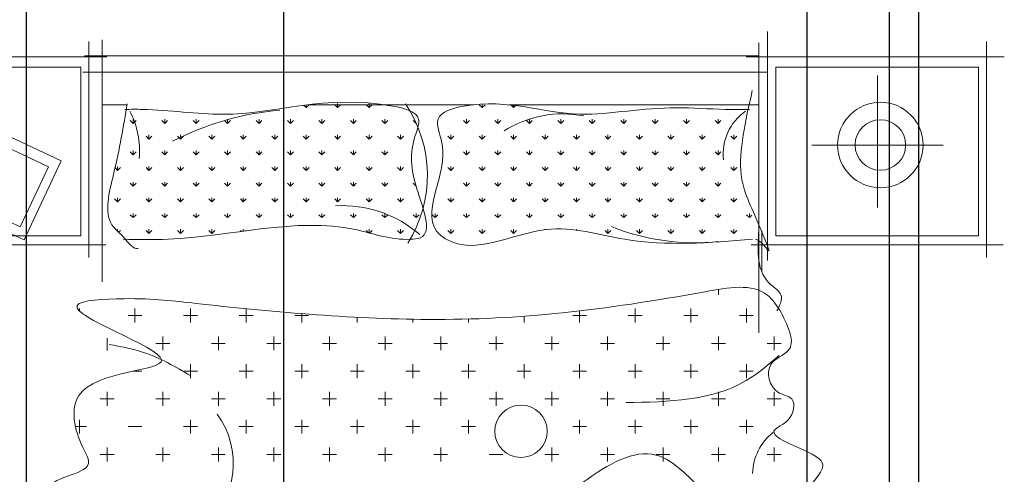
# Model space of a CAD drawing. Units: inches. Extents: x -438 to 102, y -60 to 1091.
# Tile 17 of 20: x -68 to 20, y 766 to 807. Entities that reach past the tile are written whole.
import ezdxf

# ---------------------------------------------------------------- set-up
doc = ezdxf.new("R2010")
doc.units = ezdxf.units.IN
doc.header["$MEASUREMENT"] = 0
doc.layers.add('A-ANNO-DIMS', color=217, linetype='Continuous', lineweight=18, true_color=0x93278f)
doc.layers.add('Furniture', color=7, linetype='Continuous', lineweight=15)
doc.styles.get("Standard").update_dxf_attribs({"font": 'arial.ttf'})
doc.dimstyles.get("Standard").update_dxf_attribs({"dimtxt": 8, "dimasz": 0.18, "dimexe": 0.18, "dimexo": 0.0625, "dimgap": 0.09, "dimtad": 0, "dimtih": 1, "dimtoh": 1, "dimdec": 4, "dimzin": 0, "dimdsep": 46, "dimlunit": 3, "dimtxsty": 'Standard', "dimcen": 0.09, "dimadec": 0, "dimazin": 0, "dimtfac": 1, "dimtdec": 4, "dimtofl": 0, "dimtmove": 0, "dimatfit": 3, "dimfxl": 1, "dimtolj": 1, "dimtzin": 0, "dimarcsym": 0})

# ---------------------------------------------------------------- blocks, each defined once
blk = doc.blocks.new('BED-DOUBLE-WITH-NIGHTSTANDS')
for p, q in [((30.685, 0.003), (30.685, -20.597)), ((-29.157, -22.53), (-29.157, -0.743)), ((-30.374, -20.327), (-30.374, -0.897)), ((29.898, -1.014), (29.898, -27.125)), ((50.37, -20.327), (50.37, -0.897)), ((-28.759, -2.28), (-51.984, -2.28)), ((-30.745, -2.188), (29.898, -2.188)), ((51.985, -2.28), (28.76, -2.28)), ((-31.095, -3.205), (-49.317, -3.205)), ((-31.095, -18.39), (-31.095, -3.205)), ((49.649, -3.205), (31.427, -3.205)), ((31.427, -3.205), (31.427, -18.39)), ((49.649, -18.39), (49.649, -3.205)), ((30.685, -3.641), (-30.922, -3.641)), ((40.583, -3.955), (40.583, -15.85)), ((-26.928, -6.593), (-29.157, -6.593)), ((-10.816, -6.85), (-11.024, -6.642)), ((-10.816, -6.85), (-10.551, -6.585)), ((-10.816, -6.851), (-10.816, -6.616)), ((4.241, -6.593), (-10.627, -6.593)), ((-7.988, -6.85), (-8.253, -6.585)), ((-7.988, -6.85), (-7.723, -6.585)), ((-7.987, -6.851), (-7.987, -6.476)), ((-5.159, -6.85), (-5.425, -6.585)), ((-5.159, -6.851), (-5.159, -6.476)), ((-5.159, -6.85), (-4.894, -6.585)), ((5.018, -6.85), (4.753, -6.585)), ((5.018, -6.851), (5.018, -6.53)), ((5.018, -6.85), (5.283, -6.585)), ((29.898, -6.593), (7.41, -6.593)), ((7.846, -6.85), (7.61, -6.614)), ((7.846, -6.85), (8.033, -6.663)), ((7.847, -6.851), (7.847, -6.641)), ((-26.372, -8.265), (-26.372, -7.89)), ((-23.544, -8.265), (-23.544, -7.89)), ((-20.715, -8.265), (-20.715, -7.89)), ((-17.887, -8.265), (-17.887, -7.89)), ((-15.058, -8.265), (-15.058, -7.89)), ((-12.23, -8.265), (-12.23, -7.89)), ((-9.402, -8.265), (-9.402, -7.89)), ((-6.573, -8.265), (-6.573, -7.89)), ((-3.745, -8.265), (-3.745, -7.89)), ((3.604, -8.265), (3.604, -7.89)), ((6.433, -8.265), (6.433, -7.89)), ((9.261, -8.265), (9.261, -7.89)), ((12.089, -8.265), (12.089, -7.89)), ((14.918, -8.265), (14.918, -7.89)), ((17.746, -8.265), (17.746, -7.89)), ((20.575, -8.265), (20.575, -7.89)), ((23.403, -8.265), (23.403, -7.89)), ((26.232, -8.265), (26.232, -7.89)), ((-26.373, -8.265), (-26.638, -8)), ((-26.373, -8.265), (-26.107, -8)), ((-23.544, -8.265), (-23.809, -8)), ((-23.544, -8.265), (-23.279, -8)), ((-20.716, -8.265), (-20.981, -8)), ((-20.716, -8.265), (-20.451, -8)), ((-17.887, -8.265), (-18.152, -8)), ((-17.887, -8.265), (-17.622, -8)), ((-15.059, -8.265), (-15.324, -8)), ((-15.059, -8.265), (-14.794, -8)), ((-12.23, -8.265), (-12.496, -8)), ((-12.23, -8.265), (-11.965, -8)), ((-9.402, -8.265), (-9.667, -8)), ((-9.402, -8.265), (-9.137, -8)), ((-6.574, -8.265), (-6.839, -8)), ((-6.574, -8.265), (-6.308, -8)), ((-3.745, -8.265), (-4.01, -8)), ((-3.745, -8.265), (-3.48, -8)), ((-0.917, -8.265), (-1.182, -8)), ((-0.917, -8.265), (-0.915, -8.262)), ((-0.916, -8.265), (-0.916, -8.258)), ((1.02, -8.021), (1.041, -8)), ((3.604, -8.265), (3.339, -8)), ((3.604, -8.265), (3.869, -8)), ((6.432, -8.265), (6.167, -8)), ((6.432, -8.265), (6.697, -8)), ((9.261, -8.265), (8.996, -8)), ((9.261, -8.265), (9.526, -8)), ((12.089, -8.265), (11.824, -8)), ((12.089, -8.265), (12.354, -8)), ((14.918, -8.265), (14.652, -8)), ((14.918, -8.265), (15.183, -8)), ((17.746, -8.265), (17.481, -8)), ((17.746, -8.265), (18.011, -8)), ((20.574, -8.265), (20.309, -8)), ((20.574, -8.265), (20.84, -8)), ((23.403, -8.265), (23.138, -8)), ((23.403, -8.265), (23.668, -8)), ((26.231, -8.265), (25.966, -8)), ((26.231, -8.265), (26.496, -8)), ((-32.845, -11.63), (-38.006, -9.214)), ((-24.958, -9.679), (-25.224, -9.414)), ((-24.958, -9.679), (-24.958, -9.304)), ((-24.958, -9.679), (-24.693, -9.414)), ((-22.13, -9.679), (-22.395, -9.414)), ((-22.13, -9.679), (-22.13, -9.304)), ((-22.13, -9.679), (-21.865, -9.414)), ((-19.302, -9.679), (-19.567, -9.414)), ((-19.302, -9.679), (-19.036, -9.414)), ((-19.301, -9.679), (-19.301, -9.304)), ((-16.473, -9.679), (-16.738, -9.414)), ((-16.473, -9.679), (-16.473, -9.304)), ((-16.473, -9.679), (-16.208, -9.414)), ((-13.645, -9.679), (-13.91, -9.414)), ((-13.645, -9.679), (-13.38, -9.414)), ((-13.644, -9.679), (-13.644, -9.304)), ((-10.816, -9.679), (-11.081, -9.414)), ((-10.816, -9.679), (-10.816, -9.304)), ((-10.816, -9.679), (-10.551, -9.414)), ((-7.988, -9.679), (-8.253, -9.414)), ((-7.988, -9.679), (-7.723, -9.414)), ((-7.987, -9.679), (-7.987, -9.304)), ((-5.159, -9.679), (-5.425, -9.414)), ((-5.159, -9.679), (-5.159, -9.304)), ((-5.159, -9.679), (-4.894, -9.414)), ((-2.331, -9.679), (-2.596, -9.414)), ((-2.331, -9.679), (-2.331, -9.304)), ((-2.331, -9.679), (-2.066, -9.414)), ((2.19, -9.679), (1.924, -9.414)), ((2.19, -9.679), (2.19, -9.304)), ((2.19, -9.679), (2.455, -9.414)), ((5.018, -9.679), (4.753, -9.414)), ((5.018, -9.679), (5.018, -9.304)), ((5.018, -9.679), (5.283, -9.414)), ((7.846, -9.679), (7.581, -9.414)), ((7.846, -9.679), (8.112, -9.414)), ((7.847, -9.679), (7.847, -9.304)), ((10.675, -9.679), (10.41, -9.414)), ((10.675, -9.679), (10.675, -9.304)), ((10.675, -9.679), (10.94, -9.414)), ((13.503, -9.679), (13.238, -9.414)), ((13.503, -9.679), (13.768, -9.414)), ((13.504, -9.679), (13.504, -9.304)), ((16.332, -9.679), (16.067, -9.414)), ((16.332, -9.679), (16.332, -9.304)), ((16.332, -9.679), (16.597, -9.414)), ((19.16, -9.679), (18.895, -9.414)), ((19.16, -9.679), (19.425, -9.414)), ((19.161, -9.679), (19.161, -9.304)), ((21.989, -9.679), (21.723, -9.414)), ((21.989, -9.679), (21.989, -9.304)), ((21.989, -9.679), (22.254, -9.414)), ((24.817, -9.679), (24.552, -9.414)), ((24.817, -9.679), (24.817, -9.304)), ((24.817, -9.679), (25.082, -9.414)), ((27.645, -9.679), (27.38, -9.414)), ((27.645, -9.679), (27.911, -9.414)), ((27.646, -9.679), (27.646, -9.304)), ((-34.001, -12.162), (-37.855, -10.358)), ((46.482, -10.214), (34.684, -10.214)), ((-26.373, -11.093), (-26.638, -10.828)), ((-26.373, -11.093), (-26.107, -10.828)), ((-26.372, -11.093), (-26.372, -10.718)), ((-23.544, -11.093), (-23.809, -10.828)), ((-23.544, -11.093), (-23.544, -10.718)), ((-23.544, -11.093), (-23.279, -10.828)), ((-20.716, -11.093), (-20.981, -10.828)), ((-20.716, -11.093), (-20.451, -10.828)), ((-20.715, -11.093), (-20.715, -10.718)), ((-17.887, -11.093), (-18.152, -10.828)), ((-17.887, -11.093), (-17.887, -10.718)), ((-17.887, -11.093), (-17.622, -10.828)), ((-15.059, -11.093), (-15.324, -10.828)), ((-15.059, -11.093), (-14.794, -10.828)), ((-15.058, -11.093), (-15.058, -10.718)), ((-12.23, -11.093), (-12.496, -10.828)), ((-12.23, -11.093), (-12.23, -10.718)), ((-12.23, -11.093), (-11.965, -10.828)), ((-9.402, -11.093), (-9.667, -10.828)), ((-9.402, -11.093), (-9.402, -10.718)), ((-9.402, -11.093), (-9.137, -10.828)), ((-6.574, -11.093), (-6.839, -10.828)), ((-6.574, -11.093), (-6.308, -10.828)), ((-6.573, -11.093), (-6.573, -10.718)), ((-3.745, -11.093), (-4.01, -10.828)), ((-3.745, -11.093), (-3.745, -10.718)), ((-3.745, -11.093), (-3.48, -10.828)), ((3.604, -11.093), (3.339, -10.828)), ((3.604, -11.093), (3.604, -10.718)), ((3.604, -11.093), (3.869, -10.828)), ((6.432, -11.093), (6.167, -10.828)), ((6.432, -11.093), (6.697, -10.828)), ((6.433, -11.093), (6.433, -10.718)), ((9.261, -11.093), (8.996, -10.828)), ((9.261, -11.093), (9.261, -10.718)), ((9.261, -11.093), (9.526, -10.828)), ((12.089, -11.093), (11.824, -10.828)), ((12.089, -11.093), (12.089, -10.718)), ((12.089, -11.093), (12.354, -10.828)), ((14.918, -11.093), (14.652, -10.828)), ((14.918, -11.093), (14.918, -10.718)), ((14.918, -11.093), (15.183, -10.828)), ((17.746, -11.093), (17.481, -10.828)), ((17.746, -11.093), (17.746, -10.718)), ((17.746, -11.093), (18.011, -10.828)), ((20.574, -11.093), (20.309, -10.828)), ((20.574, -11.093), (20.84, -10.828)), ((20.575, -11.093), (20.575, -10.718)), ((23.403, -11.093), (23.138, -10.828)), ((23.403, -11.093), (23.403, -10.718)), ((23.403, -11.093), (23.668, -10.828)), ((26.231, -11.093), (25.966, -10.828)), ((26.231, -11.093), (26.496, -10.828)), ((26.232, -11.093), (26.232, -10.718)), ((-36.532, -17.571), (-34.001, -12.162)), ((-36.181, -18.757), (-32.845, -11.63)), ((-27.787, -12.507), (-28.013, -12.281)), ((-27.787, -12.507), (-27.522, -12.242)), ((-27.786, -12.508), (-27.786, -12.133)), ((-24.958, -12.507), (-25.224, -12.242)), ((-24.958, -12.508), (-24.958, -12.133)), ((-24.958, -12.507), (-24.693, -12.242)), ((-22.13, -12.507), (-22.395, -12.242)), ((-22.13, -12.508), (-22.13, -12.133)), ((-22.13, -12.507), (-21.865, -12.242)), ((-19.302, -12.507), (-19.567, -12.242)), ((-19.302, -12.507), (-19.036, -12.242)), ((-19.301, -12.508), (-19.301, -12.133)), ((-16.473, -12.507), (-16.738, -12.242)), ((-16.473, -12.508), (-16.473, -12.133)), ((-16.473, -12.507), (-16.208, -12.242)), ((-13.645, -12.507), (-13.91, -12.242)), ((-13.645, -12.507), (-13.38, -12.242)), ((-13.644, -12.508), (-13.644, -12.133)), ((-10.816, -12.507), (-11.081, -12.242)), ((-10.816, -12.508), (-10.816, -12.133)), ((-10.816, -12.507), (-10.551, -12.242)), ((-7.988, -12.507), (-8.253, -12.242)), ((-7.988, -12.507), (-7.723, -12.242)), ((-7.987, -12.508), (-7.987, -12.133)), ((-5.159, -12.507), (-5.425, -12.242)), ((-5.159, -12.508), (-5.159, -12.133)), ((-5.159, -12.507), (-4.894, -12.242)), ((-2.331, -12.507), (-2.596, -12.242)), ((-2.331, -12.508), (-2.331, -12.133)), ((-2.331, -12.507), (-2.066, -12.242)), ((2.19, -12.507), (1.924, -12.242)), ((2.19, -12.508), (2.19, -12.133)), ((2.19, -12.507), (2.455, -12.242)), ((5.018, -12.507), (4.753, -12.242)), ((5.018, -12.508), (5.018, -12.133)), ((5.018, -12.507), (5.283, -12.242)), ((7.846, -12.507), (7.581, -12.242)), ((7.846, -12.507), (8.112, -12.242)), ((7.847, -12.508), (7.847, -12.133)), ((10.675, -12.507), (10.41, -12.242)), ((10.675, -12.508), (10.675, -12.133)), ((10.675, -12.507), (10.94, -12.242)), ((13.503, -12.507), (13.238, -12.242)), ((13.503, -12.507), (13.768, -12.242)), ((13.504, -12.508), (13.504, -12.133)), ((16.332, -12.507), (16.067, -12.242)), ((16.332, -12.508), (16.332, -12.133)), ((16.332, -12.507), (16.597, -12.242)), ((19.16, -12.507), (18.895, -12.242)), ((19.16, -12.507), (19.425, -12.242)), ((19.161, -12.508), (19.161, -12.133)), ((21.989, -12.507), (21.723, -12.242)), ((21.989, -12.508), (21.989, -12.133)), ((21.989, -12.507), (22.254, -12.242)), ((24.817, -12.507), (24.552, -12.242)), ((24.817, -12.508), (24.817, -12.133)), ((24.817, -12.507), (25.082, -12.242)), ((27.645, -12.507), (27.38, -12.242)), ((27.645, -12.507), (27.911, -12.242)), ((27.646, -12.508), (27.646, -12.133)), ((-26.373, -13.922), (-26.638, -13.656)), ((-26.373, -13.922), (-26.107, -13.656)), ((-26.372, -13.922), (-26.372, -13.547)), ((-23.544, -13.922), (-23.809, -13.656)), ((-23.544, -13.922), (-23.544, -13.547)), ((-23.544, -13.922), (-23.279, -13.656)), ((-20.716, -13.922), (-20.981, -13.656)), ((-20.716, -13.922), (-20.451, -13.656)), ((-20.715, -13.922), (-20.715, -13.547)), ((-17.887, -13.922), (-18.152, -13.656)), ((-17.887, -13.922), (-17.887, -13.547)), ((-17.887, -13.922), (-17.622, -13.656)), ((-15.059, -13.922), (-15.324, -13.656)), ((-15.059, -13.922), (-14.794, -13.656)), ((-15.058, -13.922), (-15.058, -13.547)), ((-12.23, -13.922), (-12.496, -13.656)), ((-12.23, -13.922), (-12.23, -13.547)), ((-12.23, -13.922), (-11.965, -13.656)), ((-9.402, -13.922), (-9.667, -13.656)), ((-9.402, -13.922), (-9.402, -13.547)), ((-9.402, -13.922), (-9.137, -13.656)), ((-6.574, -13.922), (-6.839, -13.656)), ((-6.574, -13.922), (-6.308, -13.656)), ((-6.573, -13.922), (-6.573, -13.547)), ((-3.745, -13.922), (-4.01, -13.656)), ((-3.745, -13.922), (-3.745, -13.547)), ((-3.745, -13.922), (-3.48, -13.656)), ((-0.933, -13.906), (-1.182, -13.656)), ((1.022, -13.675), (1.041, -13.656)), ((3.604, -13.922), (3.339, -13.656)), ((3.604, -13.922), (3.604, -13.547)), ((3.604, -13.922), (3.869, -13.656)), ((6.432, -13.922), (6.167, -13.656)), ((6.432, -13.922), (6.697, -13.656)), ((6.433, -13.922), (6.433, -13.547)), ((9.261, -13.922), (8.996, -13.656)), ((9.261, -13.922), (9.261, -13.547)), ((9.261, -13.922), (9.526, -13.656)), ((12.089, -13.922), (11.824, -13.656)), ((12.089, -13.922), (12.089, -13.547)), ((12.089, -13.922), (12.354, -13.656)), ((14.918, -13.922), (14.652, -13.656)), ((14.918, -13.922), (14.918, -13.547)), ((14.918, -13.922), (15.183, -13.656)), ((17.746, -13.922), (17.481, -13.656)), ((17.746, -13.922), (17.746, -13.547)), ((17.746, -13.922), (18.011, -13.656)), ((20.574, -13.922), (20.309, -13.656)), ((20.574, -13.922), (20.84, -13.656)), ((20.575, -13.922), (20.575, -13.547)), ((23.403, -13.922), (23.138, -13.656)), ((23.403, -13.922), (23.403, -13.547)), ((23.403, -13.922), (23.668, -13.656)), ((26.231, -13.922), (25.966, -13.656)), ((26.231, -13.922), (26.496, -13.656)), ((26.232, -13.922), (26.232, -13.547)), ((-27.786, -15.336), (-27.786, -14.961)), ((-24.958, -15.336), (-24.958, -14.961)), ((-22.13, -15.336), (-22.13, -14.961)), ((-19.301, -15.336), (-19.301, -14.961)), ((-16.473, -15.336), (-16.473, -14.961)), ((-13.644, -15.336), (-13.644, -14.961)), ((-10.816, -15.336), (-10.816, -14.961)), ((-7.987, -15.336), (-7.987, -14.961)), ((-5.159, -15.336), (-5.159, -14.961)), ((-2.331, -15.336), (-2.331, -14.961)), ((2.19, -15.336), (2.19, -14.961)), ((5.018, -15.336), (5.018, -14.961)), ((7.847, -15.336), (7.847, -14.961)), ((10.675, -15.336), (10.675, -14.961)), ((13.504, -15.336), (13.504, -14.961)), ((16.332, -15.336), (16.332, -14.961)), ((19.161, -15.336), (19.161, -14.961)), ((21.989, -15.336), (21.989, -14.961)), ((24.817, -15.336), (24.817, -14.961)), ((27.646, -15.336), (27.646, -14.961)), ((-40.387, -15.767), (-36.532, -17.571)), ((-27.787, -15.336), (-28.052, -15.071)), ((-27.787, -15.336), (-27.522, -15.071)), ((-24.958, -15.336), (-25.224, -15.071)), ((-24.958, -15.336), (-24.693, -15.071)), ((-22.13, -15.336), (-22.395, -15.071)), ((-22.13, -15.336), (-21.865, -15.071)), ((-19.302, -15.336), (-19.567, -15.071)), ((-19.302, -15.336), (-19.036, -15.071)), ((-16.473, -15.336), (-16.738, -15.071)), ((-16.473, -15.336), (-16.208, -15.071)), ((-13.645, -15.336), (-13.91, -15.071)), ((-13.645, -15.336), (-13.38, -15.071)), ((-10.816, -15.336), (-11.081, -15.071)), ((-10.816, -15.336), (-10.551, -15.071)), ((-7.988, -15.336), (-8.253, -15.071)), ((-7.988, -15.336), (-7.723, -15.071)), ((-5.159, -15.336), (-5.425, -15.071)), ((-5.159, -15.336), (-4.894, -15.071)), ((-2.331, -15.336), (-2.596, -15.071)), ((-2.331, -15.336), (-2.066, -15.071)), ((2.19, -15.336), (1.924, -15.071)), ((2.19, -15.336), (2.455, -15.071)), ((5.018, -15.336), (4.753, -15.071)), ((5.018, -15.336), (5.283, -15.071)), ((7.846, -15.336), (7.581, -15.071)), ((7.846, -15.336), (8.112, -15.071)), ((10.675, -15.336), (10.41, -15.071)), ((10.675, -15.336), (10.94, -15.071)), ((13.503, -15.336), (13.238, -15.071)), ((13.503, -15.336), (13.768, -15.071)), ((16.332, -15.336), (16.067, -15.071)), ((16.332, -15.336), (16.597, -15.071)), ((19.16, -15.336), (18.895, -15.071)), ((19.16, -15.336), (19.425, -15.071)), ((21.989, -15.336), (21.723, -15.071)), ((21.989, -15.336), (22.254, -15.071)), ((24.817, -15.336), (24.552, -15.071)), ((24.817, -15.336), (25.082, -15.071)), ((27.645, -15.336), (27.38, -15.071)), ((27.645, -15.336), (27.911, -15.071)), ((-41.342, -16.341), (-36.181, -18.757)), ((-26.373, -16.75), (-26.638, -16.485)), ((-26.373, -16.75), (-26.107, -16.485)), ((-26.372, -16.75), (-26.372, -16.375)), ((-23.544, -16.75), (-23.809, -16.485)), ((-23.544, -16.75), (-23.544, -16.375)), ((-23.544, -16.75), (-23.279, -16.485)), ((-20.716, -16.75), (-20.981, -16.485)), ((-20.716, -16.75), (-20.451, -16.485)), ((-20.715, -16.75), (-20.715, -16.375)), ((-17.887, -16.75), (-18.152, -16.485)), ((-17.887, -16.75), (-17.887, -16.375)), ((-17.887, -16.75), (-17.622, -16.485)), ((-15.059, -16.75), (-15.324, -16.485)), ((-15.059, -16.75), (-14.794, -16.485)), ((-15.058, -16.75), (-15.058, -16.375)), ((-12.23, -16.75), (-12.496, -16.485)), ((-12.23, -16.75), (-12.23, -16.375)), ((-12.23, -16.75), (-11.965, -16.485)), ((-9.402, -16.75), (-9.667, -16.485)), ((-9.402, -16.75), (-9.402, -16.375)), ((-9.402, -16.75), (-9.137, -16.485)), ((-6.574, -16.75), (-6.839, -16.485)), ((-6.574, -16.75), (-6.308, -16.485)), ((-6.573, -16.75), (-6.573, -16.375)), ((-3.745, -16.75), (-4.01, -16.485)), ((-3.745, -16.75), (-3.745, -16.375)), ((-3.745, -16.75), (-3.48, -16.485)), ((-0.917, -16.75), (-1.182, -16.485)), ((-0.917, -16.75), (-0.652, -16.485)), ((-0.916, -16.75), (-0.916, -16.375)), ((0.775, -16.75), (0.51, -16.485)), ((0.775, -16.75), (1.041, -16.485)), ((0.776, -16.75), (0.776, -16.375)), ((3.604, -16.75), (3.339, -16.485)), ((3.604, -16.75), (3.604, -16.375)), ((3.604, -16.75), (3.869, -16.485)), ((6.432, -16.75), (6.167, -16.485)), ((6.432, -16.75), (6.697, -16.485)), ((6.433, -16.75), (6.433, -16.375)), ((9.261, -16.75), (8.996, -16.485)), ((9.261, -16.75), (9.261, -16.375)), ((9.261, -16.75), (9.526, -16.485)), ((12.089, -16.75), (11.824, -16.485)), ((12.089, -16.75), (12.089, -16.375)), ((12.089, -16.75), (12.354, -16.485)), ((14.918, -16.75), (14.652, -16.485)), ((14.918, -16.75), (14.918, -16.375)), ((14.918, -16.75), (15.183, -16.485)), ((17.746, -16.75), (17.481, -16.485)), ((17.746, -16.75), (17.746, -16.375)), ((17.746, -16.75), (18.011, -16.485)), ((20.574, -16.75), (20.309, -16.485)), ((20.574, -16.75), (20.84, -16.485)), ((20.575, -16.75), (20.575, -16.375)), ((23.403, -16.75), (23.138, -16.485)), ((23.403, -16.75), (23.403, -16.375)), ((23.403, -16.75), (23.668, -16.485)), ((26.231, -16.75), (25.966, -16.485)), ((26.231, -16.75), (26.496, -16.485)), ((26.232, -16.75), (26.232, -16.375)), ((29.06, -16.75), (28.794, -16.485)), ((29.06, -16.75), (29.06, -16.375)), ((29.06, -16.75), (29.269, -16.541)), ((-49.317, -18.39), (-31.095, -18.39)), ((-27.786, -17.973), (-27.786, -17.79)), ((-27.69, -18.067), (-27.522, -17.899)), ((-24.958, -18.164), (-25.224, -17.899)), ((-24.958, -18.165), (-24.958, -17.79)), ((-24.958, -18.164), (-24.693, -17.899)), ((-22.13, -18.164), (-22.395, -17.899)), ((-22.13, -18.165), (-22.13, -17.79)), ((-22.13, -18.164), (-21.865, -17.899)), ((-19.302, -18.164), (-19.567, -17.899)), ((-19.302, -18.164), (-19.036, -17.899)), ((-19.301, -18.165), (-19.301, -17.79)), ((-16.65, -17.987), (-16.738, -17.899)), ((-16.473, -17.964), (-16.473, -17.79)), ((-16.242, -17.933), (-16.208, -17.899)), ((-5.211, -18.113), (-5.425, -17.899)), ((-5.159, -18.126), (-5.159, -17.79)), ((-5.129, -18.134), (-4.894, -17.899)), ((-2.331, -18.164), (-2.596, -17.899)), ((-2.331, -18.165), (-2.331, -17.79)), ((-2.331, -18.164), (-2.066, -17.899)), ((2.19, -18.164), (1.924, -17.899)), ((2.19, -18.165), (2.19, -17.79)), ((2.19, -18.164), (2.455, -17.899)), ((5.018, -18.164), (4.753, -17.899)), ((5.018, -18.165), (5.018, -17.79)), ((5.018, -18.164), (5.283, -17.899)), ((7.846, -18.164), (7.581, -17.899)), ((7.846, -18.164), (8.112, -17.899)), ((7.847, -18.165), (7.847, -17.79)), ((10.675, -17.833), (10.675, -17.79)), ((13.504, -17.877), (13.504, -17.79)), ((13.756, -17.912), (13.768, -17.899)), ((16.332, -18.164), (16.067, -17.899)), ((16.332, -18.165), (16.332, -17.79)), ((16.332, -18.164), (16.597, -17.899)), ((19.16, -18.164), (18.895, -17.899)), ((19.16, -18.164), (19.425, -17.899)), ((19.161, -18.165), (19.161, -17.79)), ((21.989, -18.164), (21.723, -17.899)), ((21.989, -18.165), (21.989, -17.79)), ((21.989, -18.164), (22.254, -17.899)), ((24.817, -18.164), (24.552, -17.899)), ((24.817, -18.165), (24.817, -17.79)), ((24.817, -18.164), (25.082, -17.899)), ((27.645, -18.164), (27.38, -17.899)), ((27.645, -18.164), (27.911, -17.899)), ((27.646, -18.165), (27.646, -17.79)), ((30.17, -21.623), (30.17, -17.936)), ((31.427, -18.39), (49.649, -18.39)), ((-51.534, -19.209), (-28.849, -19.209)), ((3.604, -19.237), (3.604, -19.204)), ((29.21, -19.209), (51.895, -19.209)), ((26.282, -23.69), (26.282, -23.209)), ((-31.218, -25.145), (-31.218, -24.94)), ((-30.593, -25.565), (-30.673, -25.565)), ((-25.593, -25.565), (-26.843, -25.565)), ((-26.218, -26.19), (-26.218, -24.94)), ((-20.593, -25.565), (-21.843, -25.565)), ((-21.218, -26.19), (-21.218, -24.94)), ((-15.593, -25.565), (-16.843, -25.565)), ((-16.218, -26.19), (-16.218, -24.951)), ((-10.593, -25.565), (-11.843, -25.565)), ((-11.218, -26.19), (-11.218, -25.392)), ((8.782, -26.19), (8.782, -25.623)), ((14.407, -25.565), (13.157, -25.565)), ((13.782, -26.19), (13.782, -25.145)), ((19.407, -25.565), (18.157, -25.565)), ((18.782, -26.19), (18.782, -24.94)), ((24.407, -25.565), (23.157, -25.565)), ((23.782, -26.19), (23.782, -24.94)), ((29.407, -25.565), (28.157, -25.565)), ((28.782, -26.19), (28.782, -24.94)), ((-6.218, -26.19), (-6.218, -25.718)), ((-1.218, -26.19), (-1.218, -25.896)), ((3.782, -26.19), (3.782, -25.874)), ((-23.718, -28.69), (-23.718, -27.44)), ((-18.718, -28.69), (-18.718, -27.44)), ((-13.718, -28.69), (-13.718, -27.44)), ((-8.718, -28.69), (-8.718, -27.44)), ((-3.718, -28.69), (-3.718, -27.44)), ((1.282, -28.69), (1.282, -27.44)), ((6.282, -28.69), (6.282, -27.44)), ((11.282, -28.69), (11.282, -27.44)), ((16.282, -28.69), (16.282, -27.44)), ((21.282, -28.69), (21.282, -27.44)), ((26.282, -28.69), (26.282, -27.44)), ((31.282, -28.69), (31.282, -27.44)), ((-28.711, -28.721), (-28.711, -27.603)), ((-23.093, -28.065), (-24.343, -28.065)), ((-18.093, -28.065), (-19.343, -28.065)), ((-13.093, -28.065), (-14.343, -28.065)), ((-8.093, -28.065), (-9.343, -28.065)), ((-3.093, -28.065), (-4.343, -28.065)), ((1.907, -28.065), (0.657, -28.065)), ((6.907, -28.065), (5.657, -28.065)), ((11.907, -28.065), (10.657, -28.065)), ((16.907, -28.065), (15.657, -28.065)), ((21.907, -28.065), (20.657, -28.065)), ((26.907, -28.065), (25.657, -28.065)), ((31.907, -28.065), (30.657, -28.065)), ((-21.218, -31.19), (-21.218, -29.94)), ((-16.218, -31.19), (-16.218, -29.94)), ((-11.218, -31.19), (-11.218, -29.94)), ((-6.218, -31.19), (-6.218, -29.94)), ((-1.218, -31.19), (-1.218, -29.94)), ((3.782, -31.19), (3.782, -29.94)), ((8.782, -31.19), (8.782, -29.94)), ((13.782, -31.19), (13.782, -29.94)), ((18.782, -31.19), (18.782, -29.94)), ((23.782, -31.19), (23.782, -29.94)), ((28.782, -31.19), (28.782, -29.94)), ((-25.593, -30.565), (-26.366, -30.565)), ((-20.593, -30.565), (-21.843, -30.565)), ((-15.593, -30.565), (-16.843, -30.565)), ((-10.593, -30.565), (-11.843, -30.565)), ((-5.593, -30.565), (-6.843, -30.565)), ((-0.593, -30.565), (-1.843, -30.565)), ((4.407, -30.565), (3.157, -30.565)), ((9.407, -30.565), (8.157, -30.565)), ((14.407, -30.565), (13.157, -30.565)), ((19.407, -30.565), (18.157, -30.565)), ((24.407, -30.565), (23.157, -30.565)), ((29.407, -30.565), (28.157, -30.565)), ((-28.718, -33.69), (-28.718, -32.44)), ((-23.718, -33.69), (-23.718, -32.44)), ((-18.718, -33.69), (-18.718, -32.44)), ((-13.718, -33.69), (-13.718, -32.44)), ((-8.718, -33.69), (-8.718, -32.44)), ((-3.718, -33.69), (-3.718, -32.44)), ((1.282, -33.69), (1.282, -32.44)), ((6.282, -33.69), (6.282, -32.44)), ((11.282, -33.69), (11.282, -32.44)), ((16.282, -33.69), (16.282, -32.44)), ((21.282, -33.69), (21.282, -32.44)), ((26.282, -33.69), (26.282, -32.44)), ((31.282, -33.69), (31.282, -32.44)), ((-28.093, -33.065), (-29.343, -33.065)), ((-23.093, -33.065), (-24.343, -33.065)), ((-18.093, -33.065), (-19.343, -33.065)), ((-13.093, -33.065), (-14.343, -33.065)), ((-8.093, -33.065), (-9.343, -33.065)), ((-3.093, -33.065), (-4.343, -33.065)), ((1.907, -33.065), (0.657, -33.065)), ((6.907, -33.065), (5.657, -33.065)), ((11.907, -33.065), (10.657, -33.065)), ((16.907, -33.065), (15.657, -33.065)), ((21.907, -33.065), (20.657, -33.065)), ((26.907, -33.065), (25.657, -33.065)), ((31.907, -33.065), (30.657, -33.065)), ((-31.218, -36.19), (-31.218, -34.94)), ((-21.218, -36.19), (-21.218, -34.94)), ((-16.218, -36.19), (-16.218, -34.94)), ((-11.218, -36.19), (-11.218, -34.94)), ((-6.218, -36.19), (-6.218, -34.94)), ((-1.218, -36.19), (-1.218, -34.94)), ((3.782, -36.19), (3.782, -34.94)), ((13.782, -36.19), (13.782, -34.94)), ((18.782, -36.19), (18.782, -34.94)), ((23.782, -36.19), (23.782, -34.94)), ((28.782, -36.19), (28.782, -34.94)), ((-30.593, -35.565), (-31.573, -35.565)), ((-25.593, -35.565), (-26.843, -35.565)), ((-20.593, -35.565), (-21.843, -35.565)), ((-15.593, -35.565), (-16.843, -35.565)), ((-10.593, -35.565), (-11.843, -35.565)), ((-5.593, -35.565), (-6.843, -35.565)), ((-0.593, -35.565), (-1.843, -35.565)), ((4.407, -35.565), (3.157, -35.565)), ((14.407, -35.565), (13.157, -35.565)), ((19.407, -35.565), (18.157, -35.565)), ((24.407, -35.565), (23.157, -35.565)), ((29.407, -35.565), (28.157, -35.565)), ((-28.093, -38.065), (-29.343, -38.065)), ((-28.718, -38.69), (-28.718, -37.44)), ((-23.093, -38.065), (-24.343, -38.065)), ((-23.718, -38.69), (-23.718, -37.44)), ((-18.093, -38.065), (-19.343, -38.065)), ((-18.718, -38.69), (-18.718, -37.44)), ((-13.093, -38.065), (-14.343, -38.065)), ((-13.718, -38.69), (-13.718, -37.44)), ((-8.093, -38.065), (-9.343, -38.065)), ((-8.718, -38.69), (-8.718, -37.44)), ((-3.093, -38.065), (-4.343, -38.065)), ((-3.718, -38.69), (-3.718, -37.44)), ((1.907, -38.065), (0.657, -38.065)), ((1.282, -38.69), (1.282, -37.44)), ((6.907, -38.065), (5.657, -38.065)), ((11.907, -38.065), (10.657, -38.065)), ((11.282, -38.69), (11.282, -37.44)), ((16.907, -38.065), (15.657, -38.065)), ((16.282, -38.69), (16.282, -37.44)), ((21.907, -38.065), (20.657, -38.065)), ((21.282, -38.69), (21.282, -37.44)), ((26.907, -38.065), (25.657, -38.065)), ((26.282, -38.69), (26.282, -37.44)), ((31.907, -38.065), (30.657, -38.065)), ((31.282, -38.69), (31.282, -37.44))]:
    blk.add_line(p, q)
for centre, radius in [((40.839, -10.214), 3.847), ((40.839, -10.214), 2.272), ((8.508, -35.984), 2.359)]:
    blk.add_circle(centre, radius)
for centre, radius, start, end in [((-10.895, -32.973), 26.004, 95.02643, 117.32994), ((-11.37, -12.946), 11.457, 327.75554, 34.13971), ((-33.344, -10.683), 7.534, 354.32477, 27.77276), ((12.254, -17.196), 9.788, 78.78839, 122.5362), ((31.354, -11.008), 4.658, 124.73446, 186.55264), ((-7.57, -26.256), 10.589, 48.87132, 93.34478), ((24.214, 1.338), 20.356, 248.18569, 275.91055), ((-24.929, -38.89), 7.557, 311.04012, 36.13845), ((34.274, -39.941), 4.944, 128.83543, 178.00379)]:
    blk.add_arc(centre, radius, start, end)
for points, knots in [([(-27.271, -18.697), (-25.925, -18.726), (-18.982, -18.878), (-10.03, -16.154), (-2.96, -18.873), (0.801, -18.493), (-1.352, -13.478), (-1.553, -10.6), (-0.228, -7.328), (-8.537, -5.307), (-15.396, -8.285), (-23.673, -6.968), (-26.611, -7), (-27.145, -7.005)], [0, 0, 0, 0, 4.049674, 20.880819, 25.932041, 26.821979, 31.217024, 36.043065, 37.533831, 40.150607, 55.448466, 62.672935, 64.278467, 64.278467, 64.278467, 64.278467]), ([(29.345, -18.697), (25.481, -19.015), (19.221, -19.531), (10.281, -16.576), (3.993, -20.465), (0.063, -17.435), (0.945, -13.788), (1.872, -10.792), (0.459, -7.428), (6.719, -5.67), (11.663, -7.909), (18.147, -7.121), (22.467, -6.733), (26.135, -7.035), (28.332, -7.013), (29.058, -7.005)], [0, 0, 0, 0, 11.502554, 18.635017, 27.654655, 28.800011, 32.595859, 36.914018, 38.927328, 41.544104, 52.009639, 56.262652, 60.661637, 65.075538, 67.252844, 67.252844, 67.252844, 67.252844]), ([(29.317, -5.316), (28.697, -8.049), (27.686, -12.508), (29.195, -15.742), (31.394, -20.84), (30.109, -18.79), (29.604, -18.697)], [0, 0, 0, 0, 7.603099, 12.404488, 14.892294, 16.432626, 16.432626, 16.432626, 16.432626]), ([(-26.912, -6.498), (-27.252, -8.516), (-27.831, -11.948), (-29.222, -16.947), (-27.139, -18.462), (-26.384, -19.61), (-25.919, -19.523)], [0, 0, 0, 0, 6.47304, 11.006869, 12.799679, 14.2185, 14.2185, 14.2185, 14.2185]), ([(29.898, -17.936), (29.784, -19.776), (29.64, -22.09), (32.269, -23.648), (31.79, -24.62), (31.531, -25.143)], [0, 0, 0, 0, 4.973031, 6.254082, 7.747585, 7.747585, 7.747585, 7.747585]), ([(31.925, -25.289), (32.572, -26.623), (33.591, -28.721), (30.294, -29.708), (31.006, -32.636), (33.349, -32.829), (32.919, -35.123), (30.078, -36.111), (33.789, -37.483), (36.776, -39.184), (33.388, -41.323), (35.068, -44.058), (26.871, -46.019), (20.992, -32.347), (2.098, -54.118), (-16.077, -50.434), (-31.165, -41.37), (-34.819, -50.791), (-35.745, -45.559), (-33.272, -44.571), (-36.072, -39.916), (-29.615, -39.911), (-31.051, -37.176), (-31.793, -35.409), (-31.667, -30.426), (-16.859, -30.756), (-35.732, -24.414), (-25.676, -23.879), (-16.82, -24.973), (2.336, -26.688), (17.46, -24.9), (30.087, -22.482), (31.544, -24.706), (31.925, -25.289)], [0, 0, 0, 0, 3.481099, 5.475811, 8.043407, 9.436812, 11.330727, 12.888379, 16.258255, 18.252967, 21.734596, 23.018392, 26.087149, 38.445812, 54.5649, 86.600283, 92.594507, 98.286547, 100.905288, 101.70342, 105.471876, 109.954916, 110.954151, 113.598333, 116.114301, 124.231953, 133.25029, 137.509046, 143.991555, 164.906349, 189.961005, 195.579007, 197.573325, 197.573325, 197.573325, 197.573325]), ([(-28.554, -28.167), (-27.498, -28.355), (-24.874, -28.821), (-22.569, -30.183), (-21.191, -30.997)], [0, 0, 0, 0, 3.194191, 7.94245, 7.94245, 7.94245, 7.94245]), ([(31.74, -29.157), (30.779, -29.979), (26.986, -33.221), (21.807, -33.325), (17.941, -33.402)], [0, 0, 0, 0, 3.737027, 14.742384, 14.742384, 14.742384, 14.742384])]:
    blk.add_open_spline(points, degree=3, knots=knots)
blk = doc.blocks.new('*D45')
at = {"layer": 'A-ANNO-DIMS', "color": 0, "lineweight": -2, "transparency": 16777216}
for p, q in [((-99.584, 615.92), (-99.584, 1079.579)), ((-99.404, 1079.399), (-59.273, 1079.399)), ((2.316, 1079.399), (-37.816, 1079.399)), ((2.496, 615.92), (2.496, 1079.579))]:
    blk.add_line(p, q, dxfattribs=at)
at = {"layer": 'A-ANNO-DIMS', "color": 0, "transparency": 16777216}
for points in [[(-99.404, 1079.429), (-99.404, 1079.369), (-99.584, 1079.399)], [(2.316, 1079.429), (2.316, 1079.369), (2.496, 1079.399)]]:
    blk.add_solid(points, dxfattribs=at)
at = {"layer": 'Defpoints', "color": 0, "transparency": 16777216}
for p in [(2.496, 1079.399), (-99.584, 615.857), (2.496, 615.857)]:
    blk.add_point(p, dxfattribs=at)
at = {"layer": 'A-ANNO-DIMS', "color": 0, "transparency": 16777216, "insert": (-48.544, 1079.399), "char_height": 8, "attachment_point": 5}
blk.add_mtext('\\A1;8\'-6"', dxfattribs=at)
blk = doc.blocks.new('*D47')
at = {"layer": 'A-ANNO-DIMS', "color": 0, "lineweight": -2, "transparency": 16777216}
for p, q in [((-67.74, 529.328), (-67.74, 1079.579)), ((-67.56, 1079.399), (-48.98, 1079.399)), ((9.731, 1079.399), (-8.849, 1079.399)), ((9.911, 529.328), (9.911, 1079.579))]:
    blk.add_line(p, q, dxfattribs=at)
at = {"layer": 'A-ANNO-DIMS', "color": 0, "transparency": 16777216}
for points in [[(-67.56, 1079.429), (-67.56, 1079.369), (-67.74, 1079.399)], [(9.731, 1079.429), (9.731, 1079.369), (9.911, 1079.399)]]:
    blk.add_solid(points, dxfattribs=at)
at = {"layer": 'Defpoints', "color": 0, "transparency": 16777216}
for p in [(9.911, 1079.399), (-67.74, 529.266), (9.911, 529.266)]:
    blk.add_point(p, dxfattribs=at)
at = {"layer": 'A-ANNO-DIMS', "color": 0, "transparency": 16777216, "insert": (-28.914, 1079.399), "char_height": 8, "attachment_point": 5}
blk.add_mtext('\\A1;6\'-5 1/2"', dxfattribs=at)
blk = doc.blocks.new('*D49')
at = {"layer": 'A-ANNO-DIMS', "color": 0, "lineweight": -2, "transparency": 16777216}
for p, q in [((-44.572, 339.857), (-44.572, 1079.579)), ((-44.392, 1079.399), (-26.894, 1079.399)), ((12.373, 1079.399), (-5.126, 1079.399)), ((12.553, 312.505), (12.553, 1079.579))]:
    blk.add_line(p, q, dxfattribs=at)
at = {"layer": 'A-ANNO-DIMS', "color": 0, "transparency": 16777216}
for points in [[(-44.392, 1079.429), (-44.392, 1079.369), (-44.572, 1079.399)], [(12.373, 1079.429), (12.373, 1079.369), (12.553, 1079.399)]]:
    blk.add_solid(points, dxfattribs=at)
at = {"layer": 'Defpoints', "color": 0, "transparency": 16777216}
for p in [(12.553, 1079.399), (-44.572, 339.795), (12.553, 312.443)]:
    blk.add_point(p, dxfattribs=at)
at = {"layer": 'A-ANNO-DIMS', "color": 0, "transparency": 16777216, "insert": (-16.01, 1079.399), "char_height": 8, "attachment_point": 5}
blk.add_mtext('\\A1;4\'-9"', dxfattribs=at)

msp = doc.modelspace()

# ---------------------------------------------------------------- block references
at = {"layer": 'Furniture'}
msp.add_blockref('BED-DOUBLE-WITH-NIGHTSTANDS', (-31.753, 805.86269), dxfattribs=at)

# ---------------------------------------------------------------- dimensions: what is measured, and where the dimension line sits
at = {"layer": 'A-ANNO-DIMS'}
for base, p1, p2, picture, middle in [((9.9115, 1079.39939), (-67.73982, 529.2655), (9.9115, 529.2655), '*D47', (-28.91416, 1079.39939)), ((2.49567, 1079.39939), (-99.58389, 615.85716), (2.49567, 615.85716), '*D45', (-48.54411, 1079.39939)), ((12.55306, 1079.39939), (-44.57214, 339.79496), (12.55306, 312.44261), '*D49', (-16.00954, 1079.39939))]:
    dim = msp.add_linear_dim(base=base, p1=p1, p2=p2, dimstyle='Standard', override={"dimdec": 1, "dimlfac": 1, "dimrnd": 0, "dimzin": 1, "dimdsep": 46, "dimlunit": 4, "dimfrac": 2}, dxfattribs=at)
    dim.commit()
    dim.dimension.update_dxf_attribs({"geometry": picture, "text_midpoint": middle})

doc.saveas('drawing.dxf')
